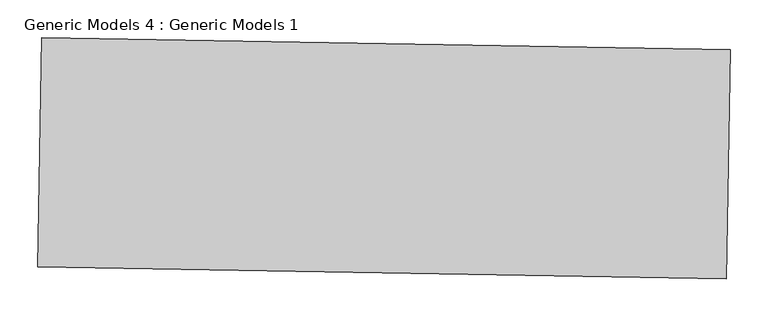
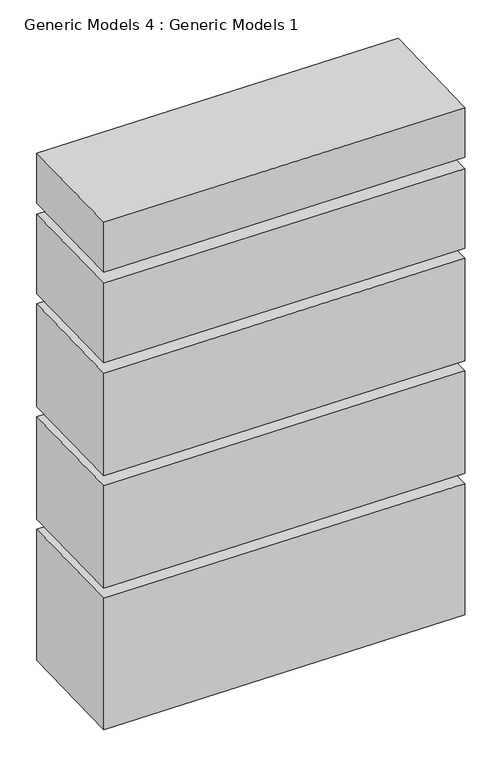
"""IFC4 building model written with IfcOpenShell, lengths in millimetres: proxy geometry, Generic Models 4 : Generic Models 1."""

from ifc_helpers import new_model, si_unit, frame, origin, place, context, project, spatial, polyline, outline, extrude, source, transform, mapped, element, save


def generic_models_4_generic_models_1_1a32cfe3(model_context):
    return source(origin(), model_context, "Body", "SweptSolid", [
        extrude(outline(polyline([(7434.7254577, -11371.6371261), (6520.4647253, -11355.6786457), (6525.7842188, -11050.9250682), (7440.0449512, -11066.8835486), (7434.7254577, -11371.6371261)])), frame((0.0, 0.0, 1263.5574996), z_axis=(0.0, 0.0, 1.0), x_axis=(1.0, 0.0, 0.0)), (0.0, 0.0, 1.0), 134.9289866),
        extrude(outline(polyline([(7434.7254577, -11371.6371261), (6520.4647253, -11355.6786457), (6525.7842188, -11050.9250682), (7440.0449512, -11066.8835486), (7434.7254577, -11371.6371261)])), frame((0.0, 0.0, 26.8864862), z_axis=(0.0, 0.0, 1.0), x_axis=(1.0, 0.0, 0.0)), (0.0, 0.0, 1.0), 354.4191875),
        extrude(outline(polyline([(7434.7254577, -11371.6371261), (6520.4647253, -11355.6786457), (6525.7842188, -11050.9250682), (7440.0449512, -11066.8835486), (7434.7254577, -11371.6371261)])), frame((0.0, 0.0, 1018.4973826), z_axis=(0.0, 0.0, 1.0), x_axis=(1.0, 0.0, 0.0)), (0.0, 0.0, 1.0), 214.5718039),
        extrude(outline(polyline([(7434.7254577, -11371.6371261), (6520.4647253, -11355.6786457), (6525.7842188, -11050.9250682), (7440.0449512, -11066.8835486), (7434.7254577, -11371.6371261)])), frame((0.0, 0.0, 713.6973826), z_axis=(0.0, 0.0, 1.0), x_axis=(1.0, 0.0, 0.0)), (0.0, 0.0, 1.0), 277.2082911),
        extrude(outline(polyline([(7434.7254577, -11371.6371261), (6520.4647253, -11355.6786457), (6525.7842188, -11050.9250682), (7440.0449512, -11066.8835486), (7434.7254577, -11371.6371261)])), frame((0.0, 0.0, 408.8973826), z_axis=(0.0, 0.0, 1.0), x_axis=(1.0, 0.0, 0.0)), (0.0, 0.0, 1.0), 277.2082911),
    ])


if __name__ == "__main__":
    model = new_model("IFC4")
    model_context = context("Model", 3, world=origin())
    ifc_project = project(units=[si_unit("LENGTHUNIT", "METRE", prefix="MILLI")], contexts=[model_context])
    site = spatial("IfcSite", under=ifc_project)
    building = spatial("IfcBuilding", under=site)
    placement = place(None, origin())
    generic_models_4_generic_models_1_shape = generic_models_4_generic_models_1_1a32cfe3(model_context)
    element("IfcBuildingElementProxy", 1, Name="Generic Models 4 : Generic Models 1", ObjectType="Generic Models 4 : Generic Models 1", at=placement, inside=building, context=model_context, shape_type="MappedRepresentation", body=[
        mapped(generic_models_4_generic_models_1_shape, transform((0.0, 0.0, 0.0), x_axis=(1.0, 0.0, 0.0), y_axis=(0.0, 1.0, 0.0), z_axis=(0.0, 0.0, 1.0))),
    ])
    save(model, "model.ifc")

# Revit data of these elements
# Element 1 (IfcBuildingElementProxy, "Generic Models 4 : Generic Models 1")
#   Materials on its faces: "Parking Stripe"
# Materials
#   "Parking Stripe": class "Paint", colour RGB 250 250 91, transparency 0, Cost = 0
